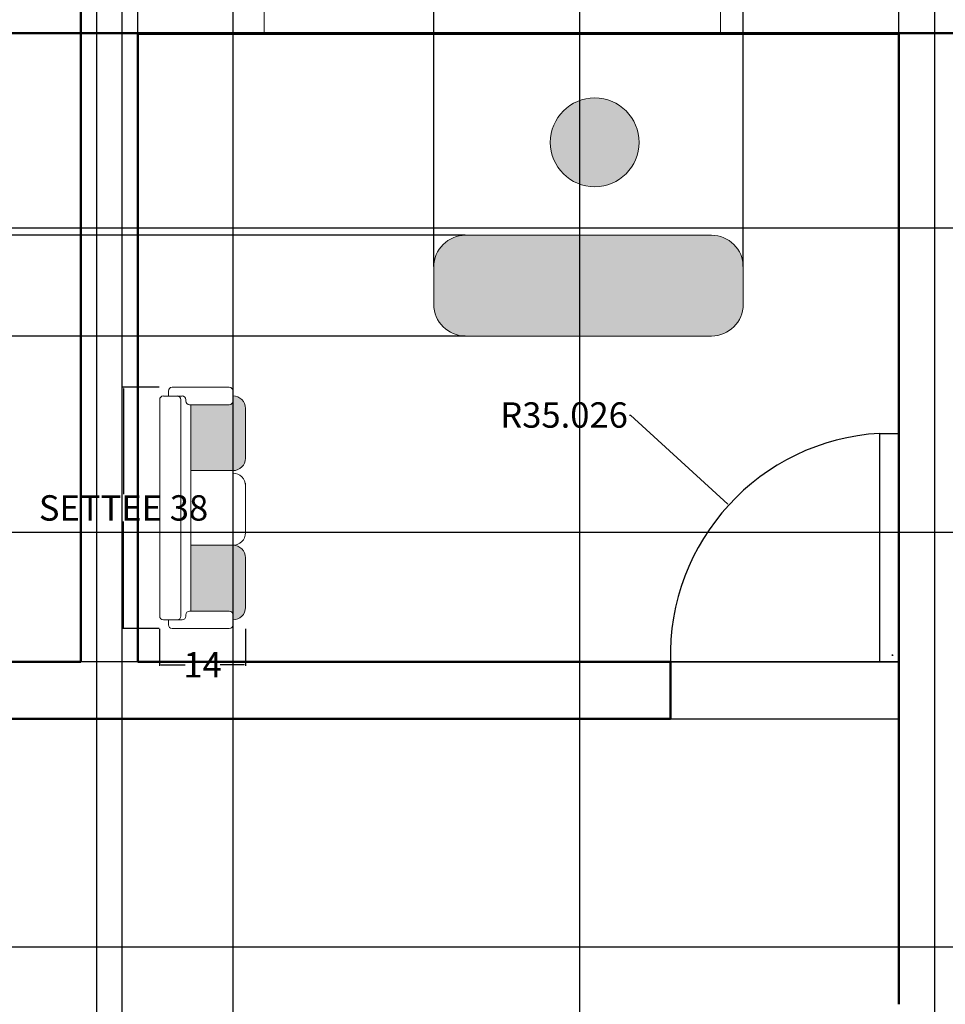
# Model space of a CAD drawing. Units: inches. Extents: x 1454 to 2136, y 626 to 1213.
# Tile 19 of 23: x 1741 to 1887, y 973 to 1128. Entities that reach past the tile are written whole.
import ezdxf

# ---------------------------------------------------------------- set-up
doc = ezdxf.new("R2010")
doc.units = ezdxf.units.IN
doc.header["$MEASUREMENT"] = 0
for name, color, linetype, lineweight in [('A-ANNO-DIMS', 2, 'Continuous', 18), ('A-DOOR', 3, 'Continuous', 25), ('A-FURN', 9, 'Continuous', 18), ('A-FURN-PATT', 252, 'Continuous', 13), ('A-GLAZ', 4, 'Continuous', 18), ('A-PLNT-PATT', 116, 'Continuous', 13), ('A-WALL', 7, 'Continuous', 50), ('sofa', 4, 'Continuous', 18)]:
    doc.layers.add(name, color=color, linetype=linetype, lineweight=lineweight)
doc.styles.get("Standard").update_dxf_attribs({"font": 'arial.ttf'})
doc.dimstyles.get("Standard").update_dxf_attribs({"dimtxt": 4, "dimasz": 0.18, "dimexe": 0.18, "dimexo": 0.0625, "dimgap": 0.09, "dimtad": 0, "dimtih": 1, "dimtoh": 1, "dimdec": 0, "dimrnd": 6, "dimzin": 0, "dimdsep": 46, "dimlunit": 3, "dimtxsty": 'Standard', "dimcen": 0.09, "dimadec": 0, "dimazin": 0, "dimtfac": 1, "dimtdec": 0, "dimtofl": 0, "dimtmove": 0, "dimatfit": 3, "dimfxl": 1, "dimtolj": 1, "dimtzin": 0, "dimarcsym": 0})

# ---------------------------------------------------------------- blocks, each defined once
blk = doc.blocks.new('A$C115861F8')
for p, q in [((0.0679, 0.6401), (0.0679, 0.6013)), ((1.7846, 0.6692), (0.097, 0.6692)), ((1.8136, 0.6401), (1.8136, 0.6013)), ((0, 0.5722), (0, 0.1261)), ((0.0679, 0.6013), (0.0291, 0.6013)), ((0.0679, 0.5334), (0.0679, 0.6013)), ((0.0679, 0.4946), (0.0679, 0.5431)), ((1.8136, 0.6013), (1.8524, 0.6013)), ((1.8136, 0.5334), (1.8136, 0.6013)), ((1.8136, 0.4946), (1.8136, 0.5431)), ((1.8815, 0.5722), (1.8815, 0.1261)), ((1.7846, 0.5043), (0.097, 0.5043)), ((0.1067, 0.4655), (0.097, 0.4655)), ((1.7749, 0.4655), (1.7846, 0.4655)), ((0.1358, 0.1261), (0.1358, 0.4364)), ((1.7458, 0.4267), (0.1358, 0.4267)), ((0.6498, 0.097), (0.6498, 0.4267)), ((1.2317, 0.097), (1.2317, 0.4267)), ((1.7458, 0.1261), (1.7458, 0.4364)), ((0.0291, 0.097), (0.1067, 0.097)), ((1.8524, 0.097), (1.7749, 0.097)), ((0.1649, 0), (0.5528, 0)), ((1.1347, 0), (0.7468, 0)), ((1.3287, 0), (1.7167, 0))]:
    blk.add_line(p, q)
for centre, radius, start, end in [((0.097, 0.6401), 0.0291, 90, 180), ((1.7846, 0.6401), 0.0291, 0, 90), ((0.0291, 0.5722), 0.0291, 90, 180), ((1.8524, 0.5722), 0.0291, 0, 90), ((0.097, 0.5334), 0.0291, 180, 270), ((0.097, 0.4946), 0.0291, 180, 270), ((0.1067, 0.4364), 0.0291, 0, 90), ((1.7749, 0.4364), 0.0291, 90, 180), ((1.7846, 0.5334), 0.0291, 270, 0), ((1.7846, 0.4946), 0.0291, 270, 0), ((0.0291, 0.1261), 0.0291, 180, 270), ((0.1649, 0.097), 0.097, 180, 270), ((0.1067, 0.1261), 0.0291, 270, 0), ((0.5528, 0.097), 0.097, 270, 0), ((0.7468, 0.097), 0.097, 180, 270), ((1.1147, 0.097), 0.097, 270, 0), ((1.3287, 0.097), 0.097, 180, 270), ((1.7167, 0.097), 0.097, 270, 0), ((1.7749, 0.1261), 0.0291, 180, 270), ((1.8524, 0.1261), 0.0291, 270, 0)]:
    blk.add_arc(centre, radius, start, end)
blk = doc.blocks.new('DOOR-LEAF-36')
blk.add_lwpolyline([(-36, 3), (0, 3), (0, 0), (-36, 0)], close=True)
blk = doc.blocks.new('*D19')
at = {"layer": 'A-ANNO-DIMS', "color": 0, "lineweight": -2, "transparency": 16777216}
for p, q in [((1762.93, 1070.55), (1757.11, 1070.55)), ((1757.29, 1070.37), (1757.29, 1053.69)), ((1757.29, 1032.69), (1757.29, 1049.37)), ((1762.93, 1032.51), (1757.11, 1032.51))]:
    blk.add_line(p, q, dxfattribs=at)
at = {"layer": 'A-ANNO-DIMS', "color": 0, "transparency": 16777216}
for points in [[(1757.26, 1070.37), (1757.32, 1070.37), (1757.29, 1070.55)], [(1757.26, 1032.69), (1757.32, 1032.69), (1757.29, 1032.51)]]:
    blk.add_solid(points, dxfattribs=at)
at = {"layer": 'Defpoints', "color": 0, "transparency": 16777216}
for p in [(1757.29, 1070.55), (1762.99, 1070.55), (1762.99, 1032.51)]:
    blk.add_point(p, dxfattribs=at)
at = {"layer": 'A-ANNO-DIMS', "color": 0, "transparency": 16777216, "insert": (1757.29, 1051.53), "char_height": 4, "attachment_point": 5}
blk.add_mtext('\\A1;SETTEE 38', dxfattribs=at)
blk = doc.blocks.new('*D20')
at = {"layer": 'A-ANNO-DIMS', "color": 0, "lineweight": -2, "transparency": 16777216}
for p, q in [((1762.99, 1032.45), (1762.99, 1026.62)), ((1776.52, 1032.45), (1776.52, 1026.62)), ((1763.17, 1026.8), (1767, 1026.8)), ((1776.34, 1026.8), (1772.52, 1026.8))]:
    blk.add_line(p, q, dxfattribs=at)
at = {"layer": 'A-ANNO-DIMS', "color": 0, "transparency": 16777216}
for points in [[(1763.17, 1026.83), (1763.17, 1026.77), (1762.99, 1026.8)], [(1776.34, 1026.83), (1776.34, 1026.77), (1776.52, 1026.8)]]:
    blk.add_solid(points, dxfattribs=at)
at = {"layer": 'Defpoints', "color": 0, "transparency": 16777216}
for p in [(1762.99, 1032.51), (1776.52, 1032.51), (1762.99, 1026.8)]:
    blk.add_point(p, dxfattribs=at)
at = {"layer": 'A-ANNO-DIMS', "color": 0, "transparency": 16777216, "insert": (1769.76, 1026.8), "char_height": 4, "attachment_point": 5}
blk.add_mtext('\\A1;14', dxfattribs=at)
blk = doc.blocks.new('*D31')
at = {"layer": 'A-ANNO-DIMS', "color": 0, "lineweight": -2, "transparency": 16777216}
for p, q in [((1759.56, 1126.34), (1759.56, 1210.46)), ((1759.74, 1210.28), (1815.24, 1210.28)), ((1879.38, 1210.28), (1823.87, 1210.28)), ((1879.56, 1126.34), (1879.56, 1210.46))]:
    blk.add_line(p, q, dxfattribs=at)
at = {"layer": 'A-ANNO-DIMS', "color": 0, "transparency": 16777216}
for points in [[(1759.74, 1210.31), (1759.74, 1210.25), (1759.56, 1210.28)], [(1879.38, 1210.31), (1879.38, 1210.25), (1879.56, 1210.28)]]:
    blk.add_solid(points, dxfattribs=at)
at = {"layer": 'Defpoints', "color": 0, "transparency": 16777216}
for p in [(1879.56, 1210.28), (1759.56, 1126.28), (1879.56, 1126.28)]:
    blk.add_point(p, dxfattribs=at)
at = {"layer": 'A-ANNO-DIMS', "color": 0, "transparency": 16777216, "insert": (1819.56, 1210.28), "char_height": 4, "attachment_point": 5}
blk.add_mtext('\\A1;120', dxfattribs=at)
blk = doc.blocks.new('*D33')
at = {"layer": 'A-ANNO-DIMS', "color": 0, "lineweight": -2, "transparency": 16777216}
for p, q in [((2032.49, 1126.28), (1462.37, 1126.28)), ((1462.55, 1126.1), (1462.55, 1056.38)), ((1462.55, 982.46), (1462.55, 1052.18)), ((2032.49, 982.28), (1462.37, 982.28))]:
    blk.add_line(p, q, dxfattribs=at)
at = {"layer": 'A-ANNO-DIMS', "color": 0, "transparency": 16777216}
for points in [[(1462.52, 1126.1), (1462.58, 1126.1), (1462.55, 1126.28)], [(1462.52, 982.46), (1462.58, 982.46), (1462.55, 982.28)]]:
    blk.add_solid(points, dxfattribs=at)
at = {"layer": 'Defpoints', "color": 0, "transparency": 16777216}
for p in [(1462.55, 1126.28), (2032.56, 1126.28), (2032.56, 982.28)]:
    blk.add_point(p, dxfattribs=at)
at = {"layer": 'A-ANNO-DIMS', "color": 0, "transparency": 16777216, "insert": (1462.55, 1054.28), "char_height": 4, "attachment_point": 5}
blk.add_mtext('\\A1;144', dxfattribs=at)
blk = doc.blocks.new('*D37')
at = {"layer": 'A-ANNO-DIMS', "color": 0, "lineweight": -2, "transparency": 16777216}
for p, q in [((1774.56, 712.34), (1774.56, 1210.46)), ((1774.74, 1210.28), (1846.74, 1210.28)), ((1927.38, 1210.28), (1855.38, 1210.28)), ((1927.56, 712.34), (1927.56, 1210.46))]:
    blk.add_line(p, q, dxfattribs=at)
at = {"layer": 'A-ANNO-DIMS', "color": 0, "transparency": 16777216}
for points in [[(1774.74, 1210.31), (1774.74, 1210.25), (1774.56, 1210.28)], [(1927.38, 1210.31), (1927.38, 1210.25), (1927.56, 1210.28)]]:
    blk.add_solid(points, dxfattribs=at)
at = {"layer": 'Defpoints', "color": 0, "transparency": 16777216}
for p in [(1927.56, 1210.28), (1774.56, 712.28), (1927.56, 712.28)]:
    blk.add_point(p, dxfattribs=at)
at = {"layer": 'A-ANNO-DIMS', "color": 0, "transparency": 16777216, "insert": (1851.06, 1210.28), "char_height": 4, "attachment_point": 5}
blk.add_mtext('\\A1;153', dxfattribs=at)
blk = doc.blocks.new('*D44')
at = {"layer": 'A-ANNO-DIMS', "color": 0, "lineweight": -2, "transparency": 16777216}
for p, q in [((1701.08, 909.11), (1701.08, 1210.46)), ((1701.26, 1210.28), (1784.96, 1210.28)), ((1885.07, 1210.28), (1801.37, 1210.28)), ((1885.25, 909.11), (1885.25, 1210.46))]:
    blk.add_line(p, q, dxfattribs=at)
at = {"layer": 'A-ANNO-DIMS', "color": 0, "transparency": 16777216}
for points in [[(1701.26, 1210.31), (1701.26, 1210.25), (1701.08, 1210.28)], [(1885.07, 1210.31), (1885.07, 1210.25), (1885.25, 1210.28)]]:
    blk.add_solid(points, dxfattribs=at)
at = {"layer": 'Defpoints', "color": 0, "transparency": 16777216}
for p in [(1885.25, 1210.28), (1701.08, 909.05), (1885.25, 909.05)]:
    blk.add_point(p, dxfattribs=at)
at = {"layer": 'A-ANNO-DIMS', "color": 0, "transparency": 16777216, "insert": (1793.16, 1210.28), "char_height": 4, "attachment_point": 5}
blk.add_mtext('\\A1;184.17', dxfattribs=at)
blk = doc.blocks.new('*D47')
at = {"layer": 'A-ANNO-DIMS', "color": 0, "lineweight": -2, "transparency": 16777216}
for p, q in [((1885.25, 909.11), (1885.25, 1210.46)), ((1885.43, 1210.28), (1899.87, 1210.28)), ((1927.38, 1210.28), (1912.94, 1210.28)), ((1927.56, 910.34), (1927.56, 1210.46))]:
    blk.add_line(p, q, dxfattribs=at)
at = {"layer": 'A-ANNO-DIMS', "color": 0, "transparency": 16777216}
for points in [[(1885.43, 1210.31), (1885.43, 1210.25), (1885.25, 1210.28)], [(1927.38, 1210.31), (1927.38, 1210.25), (1927.56, 1210.28)]]:
    blk.add_solid(points, dxfattribs=at)
at = {"layer": 'Defpoints', "color": 0, "transparency": 16777216}
for p in [(1885.25, 1210.28), (1927.56, 910.28), (1885.25, 909.05)]:
    blk.add_point(p, dxfattribs=at)
at = {"layer": 'A-ANNO-DIMS', "color": 0, "transparency": 16777216, "insert": (1906.4, 1210.28), "char_height": 4, "attachment_point": 5}
blk.add_mtext('\\A1;42.31', dxfattribs=at)
blk = doc.blocks.new('*D54')
at = {"layer": 'A-ANNO-DIMS', "color": 0, "lineweight": -2, "transparency": 16777216}
for p, q in [((1879.49, 1126.28), (1462.37, 1126.28)), ((1462.55, 1126.1), (1462.55, 1078.91)), ((1462.55, 1027.46), (1462.55, 1074.65)), ((1879.49, 1027.28), (1462.37, 1027.28))]:
    blk.add_line(p, q, dxfattribs=at)
at = {"layer": 'A-ANNO-DIMS', "color": 0, "transparency": 16777216}
for points in [[(1462.52, 1126.1), (1462.58, 1126.1), (1462.55, 1126.28)], [(1462.52, 1027.46), (1462.58, 1027.46), (1462.55, 1027.28)]]:
    blk.add_solid(points, dxfattribs=at)
at = {"layer": 'Defpoints', "color": 0, "transparency": 16777216}
for p in [(1879.56, 1126.28), (1462.55, 1027.28), (1879.56, 1027.28)]:
    blk.add_point(p, dxfattribs=at)
at = {"layer": 'A-ANNO-DIMS', "color": 0, "transparency": 16777216, "insert": (1462.55, 1076.78), "char_height": 4, "attachment_point": 5}
blk.add_mtext('\\A1;99', dxfattribs=at)
blk = doc.blocks.new('*D66')
at = {"layer": 'A-ANNO-DIMS', "color": 0, "lineweight": -2, "transparency": 16777216}
for p, q in [((1757.08, 771.01), (1757.08, 1210.46)), ((1757.26, 1210.28), (1786.34, 1210.28)), ((1829.07, 1210.28), (1799.99, 1210.28)), ((1829.25, 771.01), (1829.25, 1210.46))]:
    blk.add_line(p, q, dxfattribs=at)
at = {"layer": 'A-ANNO-DIMS', "color": 0, "transparency": 16777216}
for points in [[(1757.26, 1210.31), (1757.26, 1210.25), (1757.08, 1210.28)], [(1829.07, 1210.31), (1829.07, 1210.25), (1829.25, 1210.28)]]:
    blk.add_solid(points, dxfattribs=at)
at = {"layer": 'Defpoints', "color": 0, "transparency": 16777216}
for p in [(1829.25, 1210.28), (1757.08, 770.95), (1829.25, 770.95)]:
    blk.add_point(p, dxfattribs=at)
at = {"layer": 'A-ANNO-DIMS', "color": 0, "transparency": 16777216, "insert": (1793.16, 1210.28), "char_height": 4, "attachment_point": 5}
blk.add_mtext('\\A1;72.17', dxfattribs=at)
blk = doc.blocks.new('*D69')
at = {"layer": 'A-ANNO-DIMS', "color": 0, "lineweight": -2, "transparency": 16777216}
for p, q in [((1806.23, 1089.59), (1806.23, 1210.46)), ((1806.41, 1210.28), (1823.7, 1210.28)), ((1854.84, 1210.28), (1837.55, 1210.28)), ((1855.02, 1089.59), (1855.02, 1210.46))]:
    blk.add_line(p, q, dxfattribs=at)
at = {"layer": 'A-ANNO-DIMS', "color": 0, "transparency": 16777216}
for points in [[(1806.41, 1210.31), (1806.41, 1210.25), (1806.23, 1210.28)], [(1854.84, 1210.31), (1854.84, 1210.25), (1855.02, 1210.28)]]:
    blk.add_solid(points, dxfattribs=at)
at = {"layer": 'Defpoints', "color": 0, "transparency": 16777216}
for p in [(1855.02, 1210.28), (1806.23, 1089.52), (1855.02, 1089.52)]:
    blk.add_point(p, dxfattribs=at)
at = {"layer": 'A-ANNO-DIMS', "color": 0, "transparency": 16777216, "insert": (1830.63, 1210.28), "char_height": 4, "attachment_point": 5}
blk.add_mtext('\\A1;48.79', dxfattribs=at)
blk = doc.blocks.new('*D70')
at = {"layer": 'A-ANNO-DIMS', "color": 0, "lineweight": -2, "transparency": 16777216}
for p, q in [((1811.17, 1094.52), (1462.37, 1094.52)), ((1462.55, 1094.34), (1462.55, 1088.71)), ((1462.55, 1078.81), (1462.55, 1084.45)), ((1811.17, 1078.63), (1462.37, 1078.63))]:
    blk.add_line(p, q, dxfattribs=at)
at = {"layer": 'A-ANNO-DIMS', "color": 0, "transparency": 16777216}
for points in [[(1462.52, 1094.34), (1462.58, 1094.34), (1462.55, 1094.52)], [(1462.52, 1078.81), (1462.58, 1078.81), (1462.55, 1078.63)]]:
    blk.add_solid(points, dxfattribs=at)
at = {"layer": 'Defpoints', "color": 0, "transparency": 16777216}
for p in [(1462.55, 1094.52), (1811.23, 1094.52), (1811.23, 1078.63)]:
    blk.add_point(p, dxfattribs=at)
at = {"layer": 'A-ANNO-DIMS', "color": 0, "transparency": 16777216, "insert": (1462.55, 1086.58), "char_height": 4, "attachment_point": 5}
blk.add_mtext('\\A1;15.894', dxfattribs=at)
blk = doc.blocks.new('*D73')
at = {"layer": 'A-ANNO-DIMS', "color": 0, "lineweight": -2, "transparency": 16777216}
for p, q in [((1985.1, 1126.44), (1462.37, 1126.44)), ((1462.55, 1126.26), (1462.55, 1113.18)), ((1462.55, 1095.83), (1462.55, 1108.91)), ((1966.64, 1095.65), (1462.37, 1095.65))]:
    blk.add_line(p, q, dxfattribs=at)
at = {"layer": 'A-ANNO-DIMS', "color": 0, "transparency": 16777216}
for points in [[(1462.52, 1126.26), (1462.58, 1126.26), (1462.55, 1126.44)], [(1462.52, 1095.83), (1462.58, 1095.83), (1462.55, 1095.65)]]:
    blk.add_solid(points, dxfattribs=at)
at = {"layer": 'Defpoints', "color": 0, "transparency": 16777216}
for p in [(1985.16, 1126.44), (1462.55, 1095.65), (1966.71, 1095.65)]:
    blk.add_point(p, dxfattribs=at)
at = {"layer": 'A-ANNO-DIMS', "color": 0, "transparency": 16777216, "insert": (1462.55, 1111.04), "char_height": 4, "attachment_point": 5}
blk.add_mtext('\\A1;30.79', dxfattribs=at)
blk = doc.blocks.new('*D76')
at = {"layer": 'A-ANNO-DIMS', "color": 0, "lineweight": -2, "transparency": 16777216}
for p, q in [((1962.64, 1095.65), (1462.37, 1095.65)), ((1462.55, 1095.47), (1462.55, 1073.78)), ((1462.55, 1047.83), (1462.55, 1069.52)), ((1914.64, 1047.65), (1462.37, 1047.65))]:
    blk.add_line(p, q, dxfattribs=at)
at = {"layer": 'A-ANNO-DIMS', "color": 0, "transparency": 16777216}
for points in [[(1462.52, 1095.47), (1462.58, 1095.47), (1462.55, 1095.65)], [(1462.52, 1047.83), (1462.58, 1047.83), (1462.55, 1047.65)]]:
    blk.add_solid(points, dxfattribs=at)
at = {"layer": 'Defpoints', "color": 0, "transparency": 16777216}
for p in [(1962.71, 1095.65), (1462.55, 1047.65), (1914.71, 1047.65)]:
    blk.add_point(p, dxfattribs=at)
at = {"layer": 'A-ANNO-DIMS', "color": 0, "transparency": 16777216, "insert": (1462.55, 1071.65), "char_height": 4, "attachment_point": 5}
blk.add_mtext('\\A1;48', dxfattribs=at)
blk = doc.blocks.new('*D77')
at = {"layer": 'A-ANNO-DIMS', "color": 0, "lineweight": -2, "transparency": 16777216}
for p, q in [((1753.08, 771.01), (1753.08, 1210.46)), ((1753.26, 1210.28), (1753.6, 1210.28)), ((1756.9, 1210.28), (1756.55, 1210.28)), ((1757.08, 771.01), (1757.08, 1210.46))]:
    blk.add_line(p, q, dxfattribs=at)
at = {"layer": 'A-ANNO-DIMS', "color": 0, "transparency": 16777216}
for points in [[(1753.26, 1210.31), (1753.26, 1210.25), (1753.08, 1210.28)], [(1756.9, 1210.31), (1756.9, 1210.25), (1757.08, 1210.28)]]:
    blk.add_solid(points, dxfattribs=at)
at = {"layer": 'Defpoints', "color": 0, "transparency": 16777216}
for p in [(1757.08, 1210.28), (1753.08, 770.95), (1757.08, 770.95)]:
    blk.add_point(p, dxfattribs=at)
at = {"layer": 'A-ANNO-DIMS', "color": 0, "transparency": 16777216, "insert": (1755.08, 1210.28), "char_height": 4, "attachment_point": 5}
blk.add_mtext('\\A1;4', dxfattribs=at)
blk = doc.blocks.new('*D78')
at = {"layer": 'A-ANNO-DIMS', "color": 0, "lineweight": -2, "transparency": 16777216}
for p, q in [((1705.08, 833.11), (1705.08, 1210.46)), ((1705.26, 1210.28), (1726.04, 1210.28)), ((1752.9, 1210.28), (1732.12, 1210.28)), ((1753.08, 833.11), (1753.08, 1210.46))]:
    blk.add_line(p, q, dxfattribs=at)
at = {"layer": 'A-ANNO-DIMS', "color": 0, "transparency": 16777216}
for points in [[(1705.26, 1210.31), (1705.26, 1210.25), (1705.08, 1210.28)], [(1752.9, 1210.31), (1752.9, 1210.25), (1753.08, 1210.28)]]:
    blk.add_solid(points, dxfattribs=at)
at = {"layer": 'Defpoints', "color": 0, "transparency": 16777216}
for p in [(1753.08, 1210.28), (1705.08, 833.05), (1753.08, 833.05)]:
    blk.add_point(p, dxfattribs=at)
at = {"layer": 'A-ANNO-DIMS', "color": 0, "transparency": 16777216, "insert": (1729.08, 1210.28), "char_height": 4, "attachment_point": 5}
blk.add_mtext('\\A1;48', dxfattribs=at)
blk = doc.blocks.new('*D81')
at = {"layer": 'A-ANNO-DIMS', "color": 0, "lineweight": -2, "transparency": 16777216}
for p, q in [((1701.82, 1088.13), (1701.82, 1210.46)), ((1702, 1210.28), (1719.28, 1210.28)), ((1750.38, 1210.28), (1733.1, 1210.28)), ((1750.56, 1027.34), (1750.56, 1210.46))]:
    blk.add_line(p, q, dxfattribs=at)
at = {"layer": 'A-ANNO-DIMS', "color": 0, "transparency": 16777216}
for points in [[(1702, 1210.31), (1702, 1210.25), (1701.82, 1210.28)], [(1750.38, 1210.31), (1750.38, 1210.25), (1750.56, 1210.28)]]:
    blk.add_solid(points, dxfattribs=at)
at = {"layer": 'Defpoints', "color": 0, "transparency": 16777216}
for p in [(1701.82, 1210.28), (1701.82, 1088.07), (1750.56, 1027.28)]:
    blk.add_point(p, dxfattribs=at)
at = {"layer": 'A-ANNO-DIMS', "color": 0, "transparency": 16777216, "insert": (1726.19, 1210.28), "char_height": 4, "attachment_point": 5}
blk.add_mtext('\\A1;48.74', dxfattribs=at)
blk = doc.blocks.new('*D95')
at = {"layer": 'A-ANNO-DIMS', "color": 0, "lineweight": -2, "transparency": 16777216}
for p, q in [((1837.08, 1066.18), (1837.26, 1066.18)), ((1837.26, 1066.18), (1852.62, 1052.1)), ((1878.48, 1028.31), (1878.66, 1028.31)), ((1878.57, 1028.22), (1878.57, 1028.4))]:
    blk.add_line(p, q, dxfattribs=at)
at = {"layer": 'A-ANNO-DIMS', "color": 0, "transparency": 16777216}
blk.add_solid([(1852.64, 1052.13), (1852.59, 1052.08), (1852.75, 1051.98)], dxfattribs=at)
at = {"layer": 'Defpoints', "color": 0, "transparency": 16777216}
for p in [(1852.75, 1051.98), (1878.57, 1028.31)]:
    blk.add_point(p, dxfattribs=at)
at = {"layer": 'A-ANNO-DIMS', "color": 0, "transparency": 16777216, "insert": (1826.77, 1066.18), "char_height": 4, "attachment_point": 5}
blk.add_mtext('\\A1;R35.026', dxfattribs=at)

msp = doc.modelspace()

# ---------------------------------------------------------------- hatches: boundary and pattern name
at = {"layer": 'A-FURN-PATT'}
h = msp.add_hatch(dxfattribs=at)
h.set_pattern_fill('ESCHER', color=256)
h.paths.add_polyline_path([(1511.3761, 923.7174, 1), (1525.379, 923.7174, 1)])
h.paths.add_polyline_path([(1525.379, 816.0542, 1), (1511.3761, 816.0542, 1)])
h.paths.add_polyline_path([(1525.379, 712.7345, 1), (1511.3761, 712.7345, 1)])
h.paths.add_polyline_path([(2070.5057, 794.3402, 1), (2056.5027, 794.3402, 1)])
h.paths.add_polyline_path([(2005.868, 1014.5578, 1), (1991.8651, 1014.5578, 1)])
h.paths.add_polyline_path([(1994.0647, 1066.7584, 1), (2008.0677, 1066.7584, 1)])
h.paths.add_polyline_path([(1919.5492, 1065.3848, 1), (1933.5521, 1065.3848, 1)])
h.paths.add_polyline_path([(1936.8517, 1013.7336, 1), (1922.8488, 1013.7336, 1)])
h.paths.add_polyline_path([(1824.6062, 1109.1557, 1), (1838.6091, 1109.1557, 1)])
h = msp.add_hatch(color=256, dxfattribs=at)
h.dxf.hatch_style = 1
h.paths.add_polyline_path([(1855.0231, 1089.5248, 0.41421356), (1850.0231, 1094.5248), (1811.2288, 1094.5248, 0.41421356), (1806.2288, 1089.5248), (1806.2288, 1083.6305, 0.41421356), (1811.2288, 1078.6305), (1850.0231, 1078.6305, 0.41421356), (1855.0231, 1083.6305)])
h.paths.add_polyline_path([(1939.0638, 1089.4209), (1938.9354, 1078.7354, -0.20858653), (1943.5258, 1076.1857), (1952.7682, 1081.5837, 0.24238954)])
h.paths.add_polyline_path([(1939.0638, 1089.4209, 0.00796483), (1938.5148, 1089.4363), (1928.0643, 1089.5619), (1927.936, 1078.8906), (1938.3866, 1078.765, -0.02092855), (1938.9354, 1078.7354)])
h.paths.add_polyline_path([(1928.0643, 1089.5619), (1916.0797, 1089.706), (1916.0698, 1088.8851), (1917.241, 1088.8711, -0.41420041), (1917.7276, 1088.3726), (1917.6308, 1080.3281, -0.41422672), (1917.1324, 1079.8415), (1915.9612, 1079.8556), (1915.9573, 1079.5272, 0.41420799), (1916.4439, 1079.0288), (1927.936, 1078.8906)])
h.paths.add_polyline_path([(1917.7276, 1088.3726, 0.41420041), (1917.241, 1088.8711), (1914.9926, 1088.8981, 0.41421356), (1914.4941, 1088.4115), (1914.3974, 1080.367, 0.41421356), (1914.884, 1079.8686), (1917.1324, 1079.8415, 0.41422672), (1917.6308, 1080.3281)])
h.paths.add_polyline_path([(1928.0939, 1092.0245), (1916.6018, 1092.1627, 0.41422672), (1916.1033, 1091.6761), (1916.0797, 1089.706), (1928.0643, 1089.5619)])
h.paths.add_polyline_path([(1939.0935, 1091.8846, 0.00696804), (1938.5445, 1091.8989), (1928.0939, 1092.0245), (1928.0643, 1089.5619), (1938.5148, 1089.4363, -0.00796483), (1939.0638, 1089.4209)])
h.paths.add_polyline_path([(1939.0935, 1091.8846), (1939.0638, 1089.4209, -0.24238954), (1952.7682, 1081.5837), (1954.897, 1082.827, 0.24500473)])
h.paths.add_polyline_path([(1952.7682, 1081.5837), (1943.5258, 1076.1857, -0.16768112), (1944.8746, 1072.1191), (1944.8073, 1066.5201), (1955.4785, 1066.3918), (1955.5459, 1071.9909, 0.14799784)])
h.paths.add_polyline_path([(1954.897, 1082.827), (1952.7682, 1081.5837, -0.14799784), (1955.5459, 1071.9909), (1955.4785, 1066.3918), (1957.9412, 1066.3622), (1958.0085, 1071.9612, 0.14649407)])
h.paths.add_polyline_path([(1955.4785, 1066.3918), (1944.8073, 1066.5201), (1944.675, 1055.5205, 0.41421356), (1945.1616, 1055.0221), (1945.49, 1055.0181), (1945.5041, 1056.1893, -0.41421356), (1946.0025, 1056.6759), (1954.047, 1056.5792, -0.41421356), (1954.5336, 1056.0807), (1954.5195, 1054.9096), (1955.3404, 1054.8997)])
h.paths.add_polyline_path([(1954.5336, 1056.0807, 0.41421356), (1954.047, 1056.5792), (1946.0025, 1056.6759, 0.41421356), (1945.5041, 1056.1893), (1945.49, 1055.0181), (1945.477, 1053.9409, 0.41422115), (1945.9636, 1053.4425), (1954.0081, 1053.3458, 0.41420598), (1954.5066, 1053.8324)])
h.paths.add_polyline_path([(1957.9412, 1066.3622), (1955.4785, 1066.3918), (1955.3404, 1054.8997), (1957.3105, 1054.876, 0.41421356), (1957.8089, 1055.3626)])
h.paths.add_polyline_path([(1974.6911, 1066.3918), (1972.2285, 1066.3622), (1972.3608, 1055.3626, 0.41421356), (1972.8592, 1054.876), (1974.8293, 1054.8997)])
h.paths.add_polyline_path([(1985.3624, 1066.5201), (1974.6911, 1066.3918), (1974.8293, 1054.8997), (1975.6501, 1054.9096), (1975.6361, 1056.0807, -0.41421356), (1976.1227, 1056.5792), (1984.1672, 1056.6759, -0.41421356), (1984.6656, 1056.1893), (1984.6797, 1055.0181), (1985.008, 1055.0221, 0.41421356), (1985.4946, 1055.5205)])
h.paths.add_polyline_path([(1984.6656, 1056.1893, 0.41421356), (1984.1672, 1056.6759), (1976.1227, 1056.5792, 0.41421356), (1975.6361, 1056.0807), (1975.6631, 1053.8324, 0.41422115), (1976.1615, 1053.3458), (1984.206, 1053.4425, 0.41420597), (1984.6926, 1053.9409)])
h.paths.add_polyline_path([(1985.2951, 1072.1191, -0.16768112), (1986.6438, 1076.1857), (1977.4014, 1081.5837, 0.14799988), (1974.6238, 1071.9907), (1974.6911, 1066.3918), (1985.3624, 1066.5201)])
h.paths.add_polyline_path([(1977.4014, 1081.5837), (1975.2727, 1082.827, 0.14649407), (1972.1612, 1071.9612), (1972.2285, 1066.3622), (1974.6911, 1066.3918), (1974.6238, 1071.9907, -0.14799988)])
h.paths.add_polyline_path([(1991.1058, 1089.4209, 0.24238954), (1977.4014, 1081.5837), (1986.6438, 1076.1857, -0.20858653), (1991.2343, 1078.7354)])
h.paths.add_polyline_path([(1991.1058, 1089.4209), (1991.0762, 1091.8846, 0.24500473), (1975.2727, 1082.827), (1977.4014, 1081.5837, -0.24238954)])
h.paths.add_polyline_path([(2002.1053, 1089.5619), (1991.6547, 1089.4363, 0.00796283), (1991.1058, 1089.4209), (1991.2343, 1078.7354, -0.02092855), (1991.783, 1078.765), (2002.2336, 1078.8906)])
h.paths.add_polyline_path([(2002.0757, 1092.0245), (1991.6251, 1091.8989, 0.00696804), (1991.0762, 1091.8846), (1991.1058, 1089.4209, -0.00796283), (1991.6547, 1089.4363), (2002.1053, 1089.5619)])
h.paths.add_polyline_path([(2014.0663, 1091.6761, 0.4142004), (2013.5679, 1092.1627), (2002.0757, 1092.0245), (2002.1053, 1089.5619), (2014.09, 1089.706)])
h.paths.add_polyline_path([(2012.4421, 1088.3726, -0.41422672), (2012.9287, 1088.8711), (2014.0999, 1088.8851), (2014.09, 1089.706), (2002.1053, 1089.5619), (2002.2336, 1078.8906), (2013.7258, 1079.0288, 0.41421913), (2014.2124, 1079.5273), (2014.2084, 1079.8556), (2013.0373, 1079.8415, -0.4142004), (2012.5388, 1080.3281)])
h.paths.add_polyline_path([(1986.6438, 1024.0964), (1977.4014, 1029.4944, 0.14799988), (1974.6238, 1019.9014), (1974.6911, 1014.3025), (1985.3624, 1014.4308), (1985.2951, 1020.0298, -0.16768112)])
h.paths.add_polyline_path([(1991.1058, 1037.3316, 0.24238954), (1977.4014, 1029.4944), (1986.6438, 1024.0964, -0.20858653), (1991.2343, 1026.6461)])
h.paths.add_polyline_path([(2002.1053, 1037.4726), (1991.6547, 1037.347, 0.00796283), (1991.1058, 1037.3316), (1991.2343, 1026.6461, -0.02092855), (1991.783, 1026.6757), (2002.2336, 1026.8013)])
h.paths.add_polyline_path([(2012.4421, 1036.2833, -0.41422672), (2012.9287, 1036.7818), (2014.0999, 1036.7958), (2014.09, 1037.6167), (2002.1053, 1037.4726), (2002.2336, 1026.8013), (2013.7258, 1026.9395, 0.41421913), (2014.2124, 1027.438), (2014.2084, 1027.7663), (2013.0373, 1027.7522, -0.4142004), (2012.5388, 1028.2388)])
h.paths.add_polyline_path([(2015.6755, 1036.3222, 0.41421356), (2015.1771, 1036.8088), (2012.9287, 1036.7818, 0.41422672), (2012.4421, 1036.2833), (2012.5388, 1028.2388, 0.4142004), (2013.0373, 1027.7522), (2015.2856, 1027.7793, 0.41421356), (2015.7722, 1028.2777)])
h.paths.add_polyline_path([(1985.3624, 1014.4308), (1974.6911, 1014.3025), (1974.8293, 1002.8104), (1975.6501, 1002.8203), (1975.6361, 1003.9914, -0.41421356), (1976.1227, 1004.4899), (1984.1672, 1004.5866, -0.41421356), (1984.6656, 1004.1), (1984.6797, 1002.9288), (1985.008, 1002.9328, 0.41421356), (1985.4946, 1003.4312)])
h.paths.add_polyline_path([(1984.6656, 1004.1, 0.41421356), (1984.1672, 1004.5866), (1976.1227, 1004.4899, 0.41421356), (1975.6361, 1003.9914), (1975.6631, 1001.743, 0.41422115), (1976.1615, 1001.2564), (1984.206, 1001.3532, 0.41420598), (1984.6926, 1001.8516)])
h.paths.add_polyline_path([(1974.6911, 1014.3025), (1972.2285, 1014.2729), (1972.3608, 1003.2733, 0.41421356), (1972.8592, 1002.7867), (1974.8293, 1002.8104)])
h.paths.add_polyline_path([(1974.6238, 1019.9014, -0.14799988), (1977.4014, 1029.4944), (1975.2727, 1030.7376, 0.14649407), (1972.1612, 1019.8719), (1972.2285, 1014.2729), (1974.6911, 1014.3025)])
h.paths.add_polyline_path([(1991.1058, 1037.3316), (1991.0762, 1039.7953, 0.24500473), (1975.2727, 1030.7376), (1977.4014, 1029.4944, -0.24238954)])
h.paths.add_polyline_path([(2002.0757, 1039.9352), (1991.6251, 1039.8096, 0.00696804), (1991.0762, 1039.7953), (1991.1058, 1037.3316, -0.00796283), (1991.6547, 1037.347), (2002.1053, 1037.4726)])
h.paths.add_polyline_path([(2014.0663, 1039.5868, 0.4142004), (2013.5679, 1040.0734), (2002.0757, 1039.9352), (2002.1053, 1037.4726), (2014.09, 1037.6167)])
h.paths.add_polyline_path([(1955.5459, 1019.9016, 0.14799784), (1952.7682, 1029.4944), (1943.5258, 1024.0964, -0.16768112), (1944.8746, 1020.0298), (1944.8073, 1014.4308), (1955.4785, 1014.3025)])
h.paths.add_polyline_path([(1955.4785, 1014.3025), (1944.8073, 1014.4308), (1944.675, 1003.4312, 0.41421356), (1945.1616, 1002.9328), (1945.49, 1002.9288), (1945.5041, 1004.1, -0.41421356), (1946.0025, 1004.5866), (1954.047, 1004.4899, -0.41421356), (1954.5336, 1003.9914), (1954.5195, 1002.8203), (1955.3404, 1002.8104)])
h.paths.add_polyline_path([(1939.0638, 1037.3316), (1938.9354, 1026.6461, -0.20858653), (1943.5258, 1024.0964), (1952.7682, 1029.4944, 0.24238954)])
h.paths.add_polyline_path([(1939.0638, 1037.3316, 0.00796483), (1938.5148, 1037.347), (1928.0643, 1037.4726), (1927.936, 1026.8013), (1938.3866, 1026.6757, -0.02092855), (1938.9354, 1026.6461)])
h.paths.add_polyline_path([(1928.0643, 1037.4726), (1916.0797, 1037.6167), (1916.0698, 1036.7958), (1917.241, 1036.7818, -0.41420041), (1917.7276, 1036.2833), (1917.6308, 1028.2388, -0.41422672), (1917.1324, 1027.7522), (1915.9612, 1027.7663), (1915.9573, 1027.4379, 0.41420799), (1916.4439, 1026.9395), (1927.936, 1026.8013)])
h.paths.add_polyline_path([(1917.7276, 1036.2833, 0.41420041), (1917.241, 1036.7818), (1914.9926, 1036.8088, 0.41421356), (1914.4941, 1036.3222), (1914.3974, 1028.2777, 0.41421356), (1914.884, 1027.7793), (1917.1324, 1027.7522, 0.41422672), (1917.6308, 1028.2388)])
h.paths.add_polyline_path([(1928.0939, 1039.9352), (1916.6018, 1040.0734, 0.41422672), (1916.1033, 1039.5868), (1916.0797, 1037.6167), (1928.0643, 1037.4726)])
h.paths.add_polyline_path([(1939.0935, 1039.7953, 0.00696804), (1938.5445, 1039.8096), (1928.0939, 1039.9352), (1928.0643, 1037.4726), (1938.5148, 1037.347, -0.00796483), (1939.0638, 1037.3316)])
h.paths.add_polyline_path([(1939.0935, 1039.7953), (1939.0638, 1037.3316, -0.24238954), (1952.7682, 1029.4944), (1954.897, 1030.7376, 0.24500473)])
h.paths.add_polyline_path([(1954.897, 1030.7376), (1952.7682, 1029.4944, -0.14799784), (1955.5459, 1019.9016), (1955.4785, 1014.3025), (1957.9412, 1014.2729), (1958.0085, 1019.8719, 0.14649407)])
h.paths.add_polyline_path([(1957.9412, 1014.2729), (1955.4785, 1014.3025), (1955.3404, 1002.8104), (1957.3105, 1002.7867, 0.41421356), (1957.8089, 1003.2733)])
h.paths.add_polyline_path([(1954.5336, 1003.9914, 0.41421356), (1954.047, 1004.4899), (1946.0025, 1004.5866, 0.41421356), (1945.5041, 1004.1), (1945.49, 1002.9288), (1945.477, 1001.8516, 0.41422115), (1945.9636, 1001.3532), (1954.0081, 1001.2564, 0.41420598), (1954.5066, 1001.743)])
h.paths.add_polyline_path([(1997.553, 886.9384), (1981.0334, 886.9384), (1981.0334, 876.3409, 0.41421356), (1984.1503, 873.224), (1996.6179, 873.224, 0.41421356), (1999.7348, 876.3409), (1998.488, 876.3409, -0.41421356), (1997.553, 877.276)])
h.paths.add_polyline_path([(1981.0334, 886.9384), (1964.5139, 886.9384), (1964.5139, 877.276, -0.41421356), (1963.5788, 876.3409), (1962.3321, 876.3409, 0.41421356), (1965.449, 873.224), (1977.9165, 873.224, 0.41421356), (1981.0334, 876.3409)])
h.paths.add_polyline_path([(1964.5139, 886.9384), (1964.5139, 887.25, 0.47353022), (1963.4209, 888.1978, -0.46345458), (1962.3321, 889.1202), (1962.3321, 890.6786), (1962.3321, 892.5488), (1961.0853, 892.5488, 0.41421356), (1960.1503, 891.6137), (1960.1503, 877.276, 0.41421356), (1961.0853, 876.3409), (1963.5788, 876.3409, 0.41421356), (1964.5139, 877.276)])
h.paths.add_polyline_path([(1999.7348, 892.5488), (1999.7348, 893.7955, 0.41421356), (1998.7997, 894.7306), (1963.2672, 894.7306, 0.41421356), (1962.3321, 893.7955), (1962.3321, 892.5488), (1962.3321, 890.3669, 0.41421356), (1963.2672, 889.4319), (1998.7997, 889.4319, 0.41421356), (1999.7348, 890.3669), (1999.7348, 890.6786)])
h.paths.add_polyline_path([(2001.9166, 891.6137, 0.41421356), (2000.9815, 892.5488), (1999.7348, 892.5488), (1999.7348, 890.6786), (1999.7348, 890.3669), (1999.7348, 889.1202, -0.41421356), (1998.7997, 888.1851), (1998.488, 888.1851, 0.41421356), (1997.553, 887.25), (1997.553, 877.276, 0.41421356), (1998.488, 876.3409), (1999.7348, 876.3409), (2000.9815, 876.3409, 0.41421356), (2001.9166, 877.276)])
h.paths.add_polyline_path([(1999.7348, 889.1202), (1999.7348, 890.3669, -0.41421356), (1998.7997, 889.4319), (1963.2672, 889.4319, -0.41421356), (1962.3321, 890.3669), (1962.3321, 889.1202, 0.46345458), (1963.4209, 888.1978, -0.45647258), (1964.5139, 887.3025), (1964.5139, 886.9384), (1997.553, 886.9384), (1997.553, 887.25, -0.41421356), (1998.488, 888.1851), (1998.7997, 888.1851, 0.41421356)])
h.paths.add_polyline_path([(1540.5701, 966.1379, 0.41421356), (1538.9915, 967.7165), (1523.2061, 967.7165, 0.41421356), (1521.6275, 966.1379), (1521.6275, 964.5679, 0.41579661), (1523.2061, 962.9808), (1538.9915, 962.9808, 0.41421356), (1540.5701, 964.5594)])
h.paths.add_polyline_path([(1538.9151, 960.1995, 0.41421356), (1537.968, 961.1466), (1524.2565, 961.1466, 0.41421356), (1523.3094, 960.1995), (1523.3094, 947.859, 0.41421356), (1524.2565, 946.9119), (1537.968, 946.9119, 0.41421356), (1538.9151, 947.859)])
h.paths.add_polyline_path([(1555.8609, 960.5704, 0.41421356), (1554.9138, 961.5176), (1543.8299, 961.5176, 0.41421356), (1542.8828, 960.5704), (1542.8828, 946.859, 0.41421356), (1543.8299, 945.9119), (1554.9138, 945.9119, 0.41421356), (1555.8609, 946.859)])
h.paths.add_polyline_path([(1555.8609, 941.6364, 0.41421356), (1554.9138, 942.5835), (1543.8299, 942.5835, 0.41421356), (1542.8828, 941.6364), (1542.8828, 927.9249, 0.41421356), (1543.8299, 926.9778), (1554.9138, 926.9778, 0.41421356), (1555.8609, 927.9249)])
h.paths.add_polyline_path([(1555.8609, 922.6938, 0.41421356), (1554.9138, 923.6409), (1543.8299, 923.6409, 0.41421356), (1542.8828, 922.6938), (1542.8828, 908.9824, 0.41421356), (1543.8299, 908.0352), (1554.9138, 908.0352, 0.41421356), (1555.8609, 908.9824)])
h.paths.add_polyline_path([(1555.8609, 815.2921, 0.41421356), (1554.9138, 816.2392), (1543.8299, 816.2392, 0.41421356), (1542.8828, 815.2921), (1542.8828, 801.5806, 0.41421356), (1543.8299, 800.6335), (1554.9138, 800.6335, 0.41421356), (1555.8609, 801.5806)])
h.paths.add_polyline_path([(1555.8609, 834.2346, 0.41421356), (1554.9138, 835.1818), (1543.8299, 835.1818, 0.41421356), (1542.8828, 834.2346), (1542.8828, 820.5232, 0.41421356), (1543.8299, 819.576), (1554.9138, 819.576, 0.41421356), (1555.8609, 820.5232)])
h.paths.add_polyline_path([(1555.8609, 853.1687, 0.41421356), (1554.9138, 854.1158), (1543.8299, 854.1158, 0.41421356), (1542.8828, 853.1687), (1542.8828, 839.4572, 0.41421356), (1543.8299, 838.5101), (1554.9138, 838.5101, 0.41421356), (1555.8609, 839.4572)])
h.paths.add_polyline_path([(1538.9151, 852.7977, 0.41421356), (1537.968, 853.7448), (1524.2565, 853.7448, 0.41421356), (1523.3094, 852.7977), (1523.3094, 840.4573, 0.41421356), (1524.2565, 839.5101), (1537.968, 839.5101, 0.41421356), (1538.9151, 840.4573)])
h.paths.add_polyline_path([(1538.9151, 748.5053, 0.41421356), (1537.968, 749.4524), (1524.2565, 749.4524, 0.41421356), (1523.3094, 748.5053), (1523.3094, 736.1648, 0.41421356), (1524.2565, 735.2177), (1537.968, 735.2177, 0.41421356), (1538.9151, 736.1648)])
h.paths.add_polyline_path([(1555.8609, 748.8763, 0.41421356), (1554.9138, 749.8234), (1543.8299, 749.8234, 0.41421356), (1542.8828, 748.8763), (1542.8828, 735.1648, 0.41421356), (1543.8299, 734.2177), (1554.9138, 734.2177, 0.41421356), (1555.8609, 735.1648)])
h.paths.add_polyline_path([(1555.8609, 729.9422, 0.41421356), (1554.9138, 730.8893), (1543.8299, 730.8893, 0.41421356), (1542.8828, 729.9422), (1542.8828, 716.2308, 0.41421356), (1543.8299, 715.2836), (1554.9138, 715.2836, 0.41421356), (1555.8609, 716.2308)])
h.paths.add_polyline_path([(1555.8609, 710.9996, 0.41421356), (1554.9138, 711.9468), (1543.8299, 711.9468, 0.41421356), (1542.8828, 710.9996), (1542.8828, 697.2882, 0.41421356), (1543.8299, 696.3411), (1554.9138, 696.3411, 0.41421356), (1555.8609, 697.2882)])
h.paths.add_polyline_path([(1562.4308, 712.0232, 0.44500955), (1560.6884, 713.5932), (1559.1098, 713.5932, 0.3840739), (1557.6951, 712.0232), (1557.6951, 696.2377, 0.43158582), (1559.3667, 694.6619), (1560.9452, 694.6619, 0.39705211), (1562.4308, 696.2377)])
h.paths.add_polyline_path([(1559.2737, 713.6017, -0.41421356), (1557.6951, 715.1803), (1557.6951, 730.9658, -0.39284205), (1559.1577, 732.5401, -0.39284205), (1557.6951, 734.1143), (1557.6951, 749.8998, -0.41421356), (1559.2737, 751.4784), (1560.8522, 751.4784, -0.41421356), (1562.4308, 749.8998), (1562.4308, 734.1143, -0.39284205), (1560.9682, 732.5401, -0.39284205), (1562.4308, 730.9658), (1562.4308, 715.1803, -0.41421356), (1560.8522, 713.6017), (1559.2737, 713.5932), (1559.4375, 713.5932, 0.05204098), (1559.1098, 713.5932)])
h.paths.add_polyline_path([(1559.2737, 732.5443), (1559.2737, 732.5358), (1560.8522, 732.5358), (1560.8522, 732.5443)], flags=16)
h.paths.add_polyline_path([(1562.4308, 749.8998, 0.41421356), (1560.8522, 751.4784), (1559.2737, 751.4784, 0.41421356), (1557.6951, 749.8998), (1557.6951, 734.1143, 0.41421356), (1559.2737, 732.5358), (1559.2737, 732.5443, 0.41421356), (1557.6951, 730.9658), (1557.6951, 715.1803, 0.41421356), (1559.2737, 713.6017), (1560.8437, 713.6018, 0.41579661), (1562.4308, 715.1803), (1562.4308, 730.9658, 0.41421356), (1560.8522, 732.5443), (1560.8522, 732.5358, 0.41421356), (1562.4308, 734.1143)])
h = msp.add_hatch(color=256, dxfattribs=at)
h.dxf.hatch_style = 1
h.paths.add_polyline_path([(1776.522, 1043.6849, 0.41421356), (1774.5613, 1045.6456), (1767.8948, 1045.6456), (1767.8948, 1035.2538), (1773.9731, 1035.2538, -0.41421356), (1774.5613, 1034.6655), (1774.5613, 1033.8812, 0.41421356), (1776.522, 1035.842)])
h.paths.add_polyline_path([(1776.522, 1067.2136, 0.41421356), (1774.5613, 1069.1743), (1774.5613, 1068.39, -0.41421356), (1773.9731, 1067.8018), (1767.8948, 1067.8018), (1767.8948, 1057.4099), (1774.5613, 1057.4099, 0.41421356), (1776.522, 1059.3707)])
at = {"layer": 'A-PLNT-PATT'}
h = msp.add_hatch(dxfattribs=at)
h.set_pattern_fill('ESCHER', color=256)
h.paths.add_polyline_path([(1767.2815, 694.0009, 1), (1753.2786, 694.0009, 1)])
h.paths.add_polyline_path([(1578.6873, 1043.8029, 1), (1564.6844, 1043.8029, 1)])

# ---------------------------------------------------------------- linework, layer by layer
at = {"layer": 'A-DOOR'}
for p, q in [((1843.5563, 1027.2825), (1879.5563, 1027.2825)), ((1843.5563, 1018.2825), (1879.5563, 1018.2825))]:
    msp.add_line(p, q, dxfattribs=at)
msp.add_arc((1878.5672, 1028.3141), 35.0261, 93.291251, 181.687854, dxfattribs=at)
at = {"layer": 'A-FURN'}
msp.add_lwpolyline([(1811.2288, 1094.5248), (1850.0231, 1094.5248, -0.41421356), (1855.0231, 1089.5248), (1855.0231, 1083.6305, -0.41421356), (1850.0231, 1078.6305), (1811.2288, 1078.6305, -0.41421356), (1806.2288, 1083.6305), (1806.2288, 1089.5248, -0.41421356)], format="xyb", close=True, dxfattribs=at)
msp.add_circle((1831.6077, 1109.1557), 7.0015, dxfattribs=at)
at = {"layer": 'A-GLAZ'}
msp.add_lwpolyline([(1779.4527, 1135.2472), (1851.4527, 1135.2472), (1851.4527, 1126.2472), (1779.4527, 1126.2472)], close=True, dxfattribs=at)
at = {"layer": 'A-WALL'}
for p, q in [((1750.5563, 1171.2825), (1750.5563, 1027.2825)), ((1759.5563, 1126.2825), (1759.5563, 1027.2825)), ((1879.5563, 1126.2825), (1759.5563, 1126.2825)), ((1879.5563, 1126.2825), (1879.5563, 973.2825)), ((1750.5563, 1027.2825), (1546.5563, 1027.2825)), ((1843.5563, 1027.2825), (1759.5563, 1027.2825)), ((1843.5563, 1027.2825), (1843.5563, 1018.2825)), ((1843.5563, 1018.2825), (1537.5563, 1018.2825))]:
    msp.add_line(p, q, dxfattribs=at)

# ---------------------------------------------------------------- block references
at = {"layer": 'A-DOOR', "rotation": 90.0000000000021}
msp.add_blockref('DOOR-LEAF-36', (1879.5563, 1063.2825), dxfattribs=at)
at = {"layer": 'sofa', "xscale": 20.21645944509093, "yscale": 20.21645944509093, "zscale": 20.21645944509093, "rotation": 90}
msp.add_blockref('A$C115861F8', (1776.522, 1032.5087), dxfattribs=at)

# ---------------------------------------------------------------- dimensions: what is measured, and where the dimension line sits
at = {"layer": 'A-ANNO-DIMS'}
for base, p1, p2, override, picture, middle in [((1885.2497, 1210.2845), (1701.0763, 909.0476), (1885.2497, 909.0476), {"dimdec": 2, "dimlfac": 1, "dimrnd": 0, "dimzin": 0, "dimdsep": 46, "dimlunit": 2}, '*D44', (1793.163, 1210.2845)), ((1701.8177, 1210.2845), (1750.5563, 1027.2825), (1701.8177, 1088.0655), {"dimdec": 2, "dimlfac": 1, "dimrnd": 0, "dimzin": 0, "dimdsep": 46, "dimlunit": 2}, '*D81', (1726.187, 1210.2845)), ((1753.0763, 1210.2845), (1705.0763, 833.0476), (1753.0763, 833.0476), {"dimdec": 0, "dimlfac": 1, "dimrnd": 0, "dimzin": 0, "dimdsep": 46, "dimlunit": 2}, '*D78', (1729.0763, 1210.2845)), ((1757.0763, 1210.2845), (1753.0763, 770.9473), (1757.0763, 770.9473), {"dimdec": 0, "dimlfac": 1, "dimrnd": 0, "dimzin": 0, "dimdsep": 46, "dimlunit": 2}, '*D77', (1755.0763, 1210.2845)), ((1829.2497, 1210.2845), (1757.0763, 770.9473), (1829.2497, 770.9473), {"dimdec": 2, "dimlfac": 1, "dimrnd": 0, "dimzin": 0, "dimdsep": 46, "dimlunit": 2}, '*D66', (1793.163, 1210.2845)), ((1879.5563, 1210.2845), (1759.5563, 1126.2825), (1879.5563, 1126.2825), {"dimdec": 0, "dimlfac": 1, "dimrnd": 0, "dimzin": 0, "dimdsep": 46, "dimlunit": 2}, '*D31', (1819.5563, 1210.2845)), ((1927.5563, 1210.2845), (1774.5563, 712.2825), (1927.5563, 712.2825), {"dimdec": 0, "dimlfac": 1, "dimrnd": 0, "dimzin": 0, "dimdsep": 46, "dimlunit": 2}, '*D37', (1851.0563, 1210.2845)), ((1855.0231, 1210.2845), (1806.2288, 1089.5248), (1855.0231, 1089.5248), {"dimdec": 2, "dimlfac": 1, "dimrnd": 0, "dimzin": 0, "dimdsep": 46, "dimlunit": 2}, '*D69', (1830.626, 1210.2845)), ((1885.2497, 1210.2845), (1927.5563, 910.2825), (1885.2497, 909.0476), {"dimdec": 2, "dimlfac": 1, "dimrnd": 0, "dimzin": 0, "dimdsep": 46, "dimlunit": 2}, '*D47', (1906.403, 1210.2845))]:
    dim = msp.add_linear_dim(base=base, p1=p1, p2=p2, dimstyle='Standard', override=override, dxfattribs=at)
    dim.commit()
    dim.dimension.update_dxf_attribs({"geometry": picture, "text_midpoint": middle})
for base, p1, p2, angle, override, picture, middle in [((1462.5543, 1095.6495), (1985.1581, 1126.439), (1966.7068, 1095.6495), 90, {"dimdec": 2, "dimlfac": 1, "dimrnd": 0, "dimzin": 0, "dimdsep": 46, "dimlunit": 2}, '*D73', (1462.5543, 1111.0443)), ((1462.5543, 1126.2825), (2032.5563, 982.2825), (2032.5563, 1126.2825), 90, {"dimdec": 0, "dimlfac": 1, "dimrnd": 0, "dimzin": 0, "dimdsep": 46, "dimlunit": 2}, '*D33', (1462.5543, 1054.2825)), ((1462.5543, 1027.2825), (1879.5563, 1126.2825), (1879.5563, 1027.2825), 90, {"dimdec": 0, "dimlfac": 1, "dimrnd": 0, "dimzin": 0, "dimdsep": 46, "dimlunit": 2}, '*D54', (1462.5543, 1076.7825)), ((1462.5543, 1094.5248), (1811.2288, 1078.6305), (1811.2288, 1094.5248), 90, {"dimdec": 3, "dimlfac": 1, "dimrnd": 0, "dimzin": 0, "dimdsep": 46, "dimlunit": 2}, '*D70', (1462.5543, 1086.5777)), ((1462.5543, 1047.6495), (1962.7068, 1095.6495), (1914.7068, 1047.6495), 90, {"dimdec": 0, "dimlfac": 1, "dimrnd": 0, "dimzin": 0, "dimdsep": 46, "dimlunit": 2}, '*D76', (1462.5543, 1071.6495)), ((1762.993, 1026.803), (1776.522, 1032.5087), (1762.993, 1032.5087), 180, {"dimdec": 0, "dimlfac": 1, "dimrnd": 0, "dimzin": 0, "dimdsep": 46, "dimlunit": 2}, '*D20', (1769.7575, 1026.803))]:
    dim = msp.add_linear_dim(base=base, p1=p1, p2=p2, angle=angle, dimstyle='Standard', override=override, dxfattribs=at)
    dim.commit()
    dim.dimension.update_dxf_attribs({"geometry": picture, "text_midpoint": middle})
dim = msp.add_linear_dim(base=(1757.2873, 1070.5468), p1=(1762.993, 1032.5087), p2=(1762.993, 1070.5468), angle=90, text='SETTEE <>', dimstyle='Standard', override={"dimdec": 0, "dimlfac": 1, "dimrnd": 0, "dimzin": 0, "dimdsep": 46, "dimlunit": 2}, dxfattribs=at)
dim.commit()
dim.dimension.update_dxf_attribs({"geometry": '*D19', "text_midpoint": (1757.2873, 1051.5278)})
dim = msp.add_radius_dim(center=(1878.5672, 1028.3141), mpoint=(1852.7477, 1051.9823), dimstyle='Standard', override={"dimdec": 3, "dimlfac": 1, "dimrnd": 0, "dimzin": 0, "dimdsep": 46, "dimlunit": 2}, dxfattribs=at)
dim.commit()
dim.dimension.update_dxf_attribs({"geometry": '*D95', "text_midpoint": (1826.7705, 1066.1831), "dimtype": 164})

doc.saveas('drawing.dxf')
